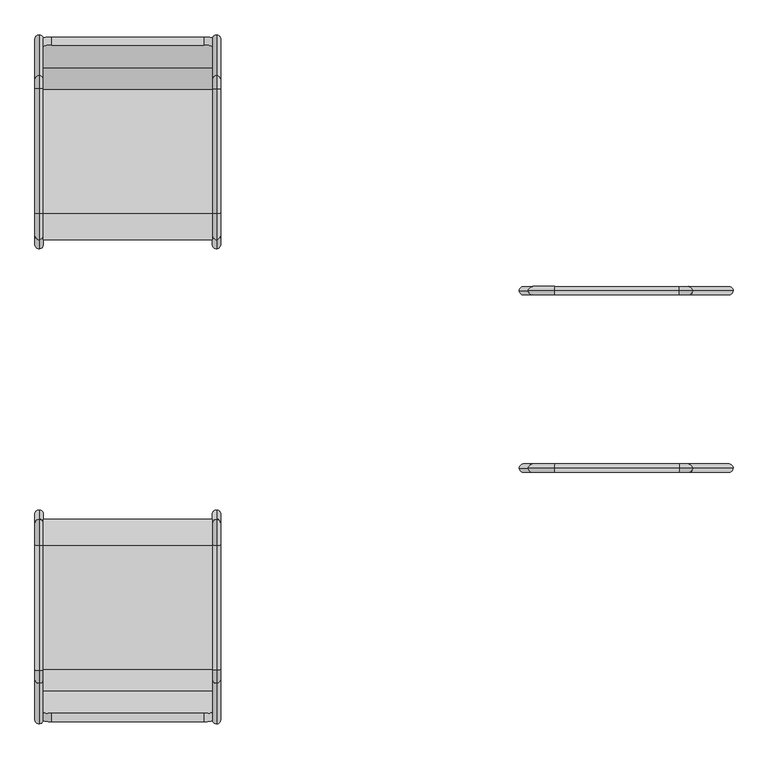
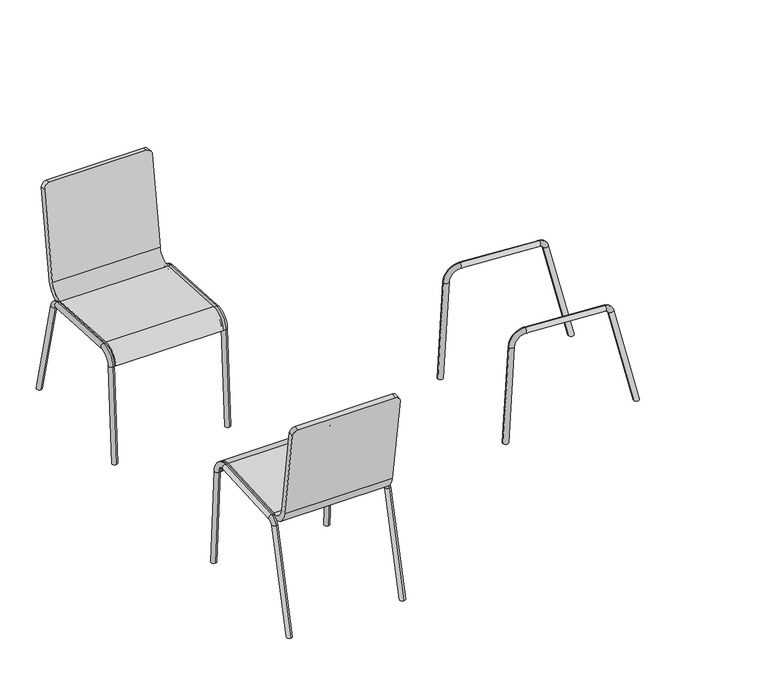
"""IFC4 building model written with IfcOpenShell, lengths in millimetres: furniture geometry."""

from ifc_helpers import new_model, si_unit, point, frame, origin, place, context, project, spatial, polyline, circle_curve, ellipse_curve, trimmed, source, transform, mapped, element, save
from ifc_brep_helpers import plane_surface, cylinder_surface, revolved_surface, advanced_brep


def furniture_c31c7c6f(model_context):
    return source(origin(), model_context, "Body", "AdvancedBrep", [
        advanced_brep(
        [(-273.9849702, -804.6938637, 0.0), (-273.9849702, -825.3061363, 0.0), (-263.9849702, -323.0385228, 0.0), (-273.9849702, -333.0554387, 0.0), (-283.9849702, -323.0385228, 0.0), (-273.9849702, -709.1722272, 383.1163586), (-273.9849702, -728.5781417, 387.9547965), (-273.9849702, -696.6509897, 414.4284246), (-273.9849702, -695.489162, 394.4621992), (-273.9849702, -398.2489468, 431.792335), (-273.9849702, -397.0871192, 411.8261096), (-273.9849702, -334.8647877, 375.3791418), (-273.9849702, -354.8310131, 374.2173141), (-273.9849702, -313.0554101, 0.5809138)],
        [
            (0, 1, ellipse_curve(frame((-273.9849702, -815.0, 0.0), z_axis=(0.0, 0.0, -1.0), x_axis=(0.0, -1.0, 0.0)), 10.3061363, 10.0)),
            (1, 0, ellipse_curve(frame((-273.9849702, -815.0, 0.0), z_axis=(0.0, 0.0, -1.0), x_axis=(0.0, -1.0, 0.0)), 10.3061363, 10.0)),
            (2, 3, ellipse_curve(frame((-273.9849702, -323.0385228, 0.0), z_axis=(0.0, 0.0, -1.0), x_axis=(0.0, -1.0, 0.0)), 10.0169159, 10.0)),
            (3, 4, ellipse_curve(frame((-273.9849702, -323.0385228, 0.0), z_axis=(0.0, 0.0, -1.0), x_axis=(0.0, -1.0, 0.0)), 10.0169159, 10.0)),
            (4, 2),
            (5, 0),
            (1, 6),
            (6, 5, circle_curve(frame((-273.9849702, -718.8751844, 385.5355776), z_axis=(0.0, -0.24192189559966623, -0.9702957262759968), x_axis=(0.0, -0.9702957262759968, 0.24192189559966623)), 10.0)),
            (5, 6, circle_curve(frame((-273.9849702, -718.8751844, 385.5355776), z_axis=(0.0, -0.24192189559966623, -0.9702957262759968), x_axis=(0.0, -0.9702957262759968, 0.24192189559966623)), 10.0)),
            (6, 7, circle_curve(frame((-273.9849702, -694.6177913, 379.4875302), z_axis=(-1.0, 0.0, 0.0), x_axis=(0.0, -0.9702957262759969, 0.2419218955996659)), 35.0)),
            (7, 8, circle_curve(frame((-273.9849702, -696.0700758, 404.4453119), z_axis=(0.0, -0.9983112697039765, -0.05809138302738456), x_axis=(0.0, -0.05809138302738456, 0.9983112697039765)), 10.0)),
            (8, 5, circle_curve(frame((-273.9849702, -694.6177913, 379.4875302), z_axis=(1.0, 0.0, 0.0), x_axis=(0.0, -0.9702957262759969, 0.2419218955996659)), 15.0)),
            (8, 7, circle_curve(frame((-273.9849702, -696.0700758, 404.4453119), z_axis=(0.0, -0.998311269703977, -0.05809138302737549), x_axis=(0.0, -0.05809138302737549, 0.998311269703977)), 10.0)),
            (7, 9),
            (9, 10, circle_curve(frame((-273.9849702, -397.668033, 421.8092223), z_axis=(0.0, -0.9983112697039764, -0.058091383027386895), x_axis=(0.0, -0.058091383027386895, 0.9983112697039764)), 10.0)),
            (10, 8),
            (10, 9, circle_curve(frame((-273.9849702, -397.668033, 421.8092223), z_axis=(0.0, -0.9983112697039764, -0.058091383027386895), x_axis=(0.0, -0.058091383027386895, 0.9983112697039764)), 10.0)),
            (9, 11, circle_curve(frame((-273.9849702, -394.7634639, 371.8936588), z_axis=(-1.0, 0.0, 0.0), x_axis=(0.0, -0.05809138302738633, 0.9983112697039764)), 60.0)),
            (11, 12, circle_curve(frame((-273.9849702, -344.8479004, 374.7982279), z_axis=(0.0, -0.05809138302739081, 0.9983112697039762), x_axis=(0.0, 0.9983112697039762, 0.05809138302739081)), 10.0)),
            (12, 10, circle_curve(frame((-273.9849702, -394.7634639, 371.8936588), z_axis=(1.0, 0.0, 0.0), x_axis=(0.0, -0.05809138302738633, 0.9983112697039764)), 40.0)),
            (12, 11, circle_curve(frame((-273.9849702, -344.8479004, 374.7982279), z_axis=(0.0, -0.05809138302739125, 0.9983112697039761), x_axis=(0.0, 0.9983112697039761, 0.05809138302739125)), 10.0)),
            (4, 13, circle_curve(frame((-273.9849702, -323.0385228, 0.0), z_axis=(0.0, 0.058091383027392335, -0.9983112697039761), x_axis=(0.0, 0.9983112697039761, 0.058091383027392335)), 10.0)),
            (13, 2, circle_curve(frame((-273.9849702, -323.0385228, 0.0), z_axis=(0.0, 0.058091383027392335, -0.9983112697039761), x_axis=(0.0, 0.9983112697039761, 0.058091383027392335)), 10.0)),
            (11, 13),
            (3, 12),
        ],
        [
            plane_surface(frame((-236.564671, -850.4463822, 0.0), z_axis=(0.0, 0.0, -1.0), x_axis=(-1.0, 0.0, 0.0))),
            cylinder_surface(frame((-273.9849702, -817.6101503, -10.4687411), z_axis=(0.0, -0.24192189559966623, -0.9702957262759968), x_axis=(0.0, -0.9702957262759968, 0.24192189559966623)), 10.0),
            revolved_surface(trimmed(ellipse_curve(frame((-273.9849702, -718.8751844, 385.5355776), z_axis=(0.0, 0.2419218955996659, 0.9702957262759969), x_axis=(0.0, -0.9702957262759969, 0.2419218955996659)), 10.0, 10.0), [point((-273.9849702, -709.1722272, 383.1163586))], [point((-273.9849702, -728.5781417, 387.9547965))], True, "CARTESIAN"), (-293.9849702, -694.6177913, 379.4875302), (1.0, 0.0, 0.0)),
            revolved_surface(trimmed(ellipse_curve(frame((-273.9849702, -718.8751844, 385.5355776), z_axis=(0.0, 0.2419218955996659, 0.9702957262759969), x_axis=(0.0, -0.9702957262759969, 0.2419218955996659)), 10.0, 10.0), [point((-273.9849702, -728.5781417, 387.9547965))], [point((-273.9849702, -709.1722272, 383.1163586))], True, "CARTESIAN"), (-293.9849702, -694.6177913, 379.4875302), (1.0, 0.0, 0.0)),
            cylinder_surface(frame((-273.9849702, -696.0700758, 404.4453119), z_axis=(0.0, -0.9983112697039764, -0.058091383027386895), x_axis=(0.0, -0.058091383027386895, 0.9983112697039764)), 10.0),
            revolved_surface(trimmed(ellipse_curve(frame((-273.9849702, -397.668033, 421.8092223), z_axis=(0.0, 0.9983112697039764, 0.05809138302738631), x_axis=(0.0, -0.05809138302738631, 0.9983112697039764)), 10.0, 10.0), [point((-273.9849702, -397.0871192, 411.8261096))], [point((-273.9849702, -398.2489468, 431.792335))], True, "CARTESIAN"), (-293.9849702, -394.7634639, 371.8936588), (1.0, 0.0, 0.0)),
            revolved_surface(trimmed(ellipse_curve(frame((-273.9849702, -397.668033, 421.8092223), z_axis=(0.0, 0.9983112697039764, 0.05809138302738631), x_axis=(0.0, -0.05809138302738631, 0.9983112697039764)), 10.0, 10.0), [point((-273.9849702, -398.2489468, 431.792335))], [point((-273.9849702, -397.0871192, 411.8261096))], True, "CARTESIAN"), (-293.9849702, -394.7634639, 371.8936588), (1.0, 0.0, 0.0)),
            plane_surface(frame((-293.9849702, -323.0385228, 0.0), z_axis=(0.0, 0.058091383027392335, -0.9983112697039761), x_axis=(1.0, 0.0, 0.0))),
            cylinder_surface(frame((-273.9849702, -344.8479004, 374.7982279), z_axis=(0.0, -0.058091383027392335, 0.9983112697039761), x_axis=(0.0, 0.9983112697039761, 0.058091383027392335)), 10.0),
        ],
        [
            (0, [[1, 2]]),
            (0, [[3, 4, 5]]),
            (1, [[6, -2, 7, 8]]),
            (1, [[-7, -1, -6, 9]]),
            (2, [[10, 11, 12, -8]]),
            (3, [[-12, 13, -10, -9]]),
            (4, [[14, 15, 16, -11]]),
            (4, [[-16, 17, -14, -13]]),
            (5, [[18, 19, 20, -15]]),
            (6, [[-20, 21, -18, -17]]),
            (7, [[-5, 22, 23]]),
            (8, [[24, -22, -4, 25, -19]]),
            (8, [[-25, -3, -23, -24, -21]]),
        ],
    ),
        advanced_brep(
        [(-689.1443717, -323.0385228, 0.0), (-709.1443717, -323.0385228, 0.0), (-699.1443717, -313.0554101, 0.5809138), (-699.1443717, -709.1722272, 383.1163586), (-699.1443717, -804.6938637, 0.0), (-699.1443717, -825.3061363, 0.0), (-699.1443717, -728.5781417, 387.9547965), (-699.1443717, -333.0554387, 0.0), (-699.1443717, -696.6509897, 414.4284246), (-699.1443717, -398.2489468, 431.792335), (-699.1443717, -397.0871192, 411.8261096), (-699.1443717, -695.489162, 394.4621992), (-699.1443717, -334.8647877, 375.3791418), (-699.1443717, -354.8310131, 374.2173141)],
        [
            (0, 1),
            (1, 2, circle_curve(frame((-699.1443717, -323.0385228, 0.0), z_axis=(0.0, 0.058091383027392335, -0.9983112697039761), x_axis=(0.0, 0.9983112697039761, 0.058091383027392335)), 10.0)),
            (2, 0, circle_curve(frame((-699.1443717, -323.0385228, 0.0), z_axis=(0.0, 0.058091383027392335, -0.9983112697039761), x_axis=(0.0, 0.9983112697039761, 0.058091383027392335)), 10.0)),
            (3, 4),
            (4, 5, ellipse_curve(frame((-699.1443717, -815.0, 0.0), z_axis=(0.0, 0.0, 1.0), x_axis=(0.0, -1.0, 0.0)), 10.3061363, 10.0)),
            (5, 6),
            (6, 3, circle_curve(frame((-699.1443717, -718.8751844, 385.5355776), z_axis=(0.0, -0.24192189559966623, -0.9702957262759968), x_axis=(0.0, -0.9702957262759968, 0.24192189559966623)), 10.0)),
            (5, 4, ellipse_curve(frame((-699.1443717, -815.0, 0.0), z_axis=(0.0, 0.0, 1.0), x_axis=(0.0, -1.0, 0.0)), 10.3061363, 10.0)),
            (3, 6, circle_curve(frame((-699.1443717, -718.8751844, 385.5355776), z_axis=(0.0, -0.24192189559966623, -0.9702957262759968), x_axis=(0.0, -0.9702957262759968, 0.24192189559966623)), 10.0)),
            (0, 7, ellipse_curve(frame((-699.1443717, -323.0385228, 0.0), z_axis=(0.0, 0.0, -1.0), x_axis=(0.0, -1.0, 0.0)), 10.0169159, 10.0)),
            (7, 1, ellipse_curve(frame((-699.1443717, -323.0385228, 0.0), z_axis=(0.0, 0.0, -1.0), x_axis=(0.0, -1.0, 0.0)), 10.0169159, 10.0)),
            (8, 9),
            (9, 10, circle_curve(frame((-699.1443717, -397.668033, 421.8092223), z_axis=(0.0, -0.9983112697039764, -0.058091383027386895), x_axis=(0.0, -0.058091383027386895, 0.9983112697039764)), 10.0)),
            (10, 11),
            (11, 8, circle_curve(frame((-699.1443717, -696.0700758, 404.4453119), z_axis=(0.0, 0.9983112697039764, 0.058091383027386895), x_axis=(0.0, -0.058091383027386895, 0.9983112697039764)), 10.0)),
            (10, 9, circle_curve(frame((-699.1443717, -397.668033, 421.8092223), z_axis=(0.0, -0.9983112697039764, -0.058091383027386895), x_axis=(0.0, -0.058091383027386895, 0.9983112697039764)), 10.0)),
            (8, 11, circle_curve(frame((-699.1443717, -696.0700758, 404.4453119), z_axis=(0.0, 0.9983112697039764, 0.058091383027386895), x_axis=(0.0, -0.058091383027386895, 0.9983112697039764)), 10.0)),
            (9, 12, circle_curve(frame((-699.1443717, -394.7634639, 371.8936588), z_axis=(-1.0, 0.0, 0.0), x_axis=(0.0, -0.05809138302738633, 0.9983112697039764)), 60.0)),
            (12, 13, circle_curve(frame((-699.1443717, -344.8479004, 374.7982279), z_axis=(0.0, -0.058091383027391474, 0.9983112697039761), x_axis=(0.0, 0.9983112697039761, 0.058091383027391474)), 10.0)),
            (13, 10, circle_curve(frame((-699.1443717, -394.7634639, 371.8936588), z_axis=(1.0, 0.0, 0.0), x_axis=(0.0, -0.05809138302738633, 0.9983112697039764)), 40.0)),
            (13, 12, circle_curve(frame((-699.1443717, -344.8479004, 374.7982279), z_axis=(0.0, -0.05809138302739081, 0.9983112697039762), x_axis=(0.0, 0.9983112697039762, 0.05809138302739081)), 10.0)),
            (12, 2),
            (7, 13),
            (6, 8, circle_curve(frame((-699.1443717, -694.6177913, 379.4875302), z_axis=(-1.0, 0.0, 0.0), x_axis=(0.0, -0.9702957262759969, 0.2419218955996659)), 35.0)),
            (11, 3, circle_curve(frame((-699.1443717, -694.6177913, 379.4875302), z_axis=(1.0, 0.0, 0.0), x_axis=(0.0, -0.9702957262759969, 0.2419218955996659)), 15.0)),
        ],
        [
            plane_surface(frame((-679.1443717, -323.0385228, 0.0), z_axis=(0.0, 0.058091383027392335, -0.9983112697039761), x_axis=(-1.0, 0.0, 0.0))),
            cylinder_surface(frame((-699.1443717, -817.6101503, -10.4687411), z_axis=(0.0, -0.24192189559966623, -0.9702957262759968), x_axis=(0.0, -0.9702957262759968, 0.24192189559966623)), 10.0),
            plane_surface(frame((-236.564671, -850.4463822, 0.0), z_axis=(0.0, 0.0, -1.0), x_axis=(-1.0, 0.0, 0.0))),
            cylinder_surface(frame((-699.1443717, -696.0700758, 404.4453119), z_axis=(0.0, -0.9983112697039764, -0.058091383027386895), x_axis=(0.0, -0.058091383027386895, 0.9983112697039764)), 10.0),
            revolved_surface(trimmed(ellipse_curve(frame((-699.1443717, -397.668033, 421.8092223), z_axis=(0.0, 0.9983112697039764, 0.05809138302738631), x_axis=(0.0, -0.05809138302738631, 0.9983112697039764)), 10.0, 10.0), [point((-699.1443717, -397.0871192, 411.8261096))], [point((-699.1443717, -398.2489468, 431.792335))], True, "CARTESIAN"), (-679.1443717, -394.7634639, 371.8936588), (1.0, 0.0, 0.0)),
            revolved_surface(trimmed(ellipse_curve(frame((-699.1443717, -397.668033, 421.8092223), z_axis=(0.0, 0.9983112697039764, 0.05809138302738631), x_axis=(0.0, -0.05809138302738631, 0.9983112697039764)), 10.0, 10.0), [point((-699.1443717, -398.2489468, 431.792335))], [point((-699.1443717, -397.0871192, 411.8261096))], True, "CARTESIAN"), (-679.1443717, -394.7634639, 371.8936588), (1.0, 0.0, 0.0)),
            cylinder_surface(frame((-699.1443717, -344.8479004, 374.7982279), z_axis=(0.0, -0.058091383027392335, 0.9983112697039761), x_axis=(0.0, 0.9983112697039761, 0.058091383027392335)), 10.0),
            revolved_surface(trimmed(ellipse_curve(frame((-699.1443717, -718.8751844, 385.5355776), z_axis=(0.0, 0.2419218955996659, 0.9702957262759969), x_axis=(0.0, -0.9702957262759969, 0.2419218955996659)), 10.0, 10.0), [point((-699.1443717, -709.1722272, 383.1163586))], [point((-699.1443717, -728.5781417, 387.9547965))], True, "CARTESIAN"), (-679.1443717, -694.6177913, 379.4875302), (1.0, 0.0, 0.0)),
            revolved_surface(trimmed(ellipse_curve(frame((-699.1443717, -718.8751844, 385.5355776), z_axis=(0.0, 0.2419218955996659, 0.9702957262759969), x_axis=(0.0, -0.9702957262759969, 0.2419218955996659)), 10.0, 10.0), [point((-699.1443717, -728.5781417, 387.9547965))], [point((-699.1443717, -709.1722272, 383.1163586))], True, "CARTESIAN"), (-679.1443717, -694.6177913, 379.4875302), (1.0, 0.0, 0.0)),
        ],
        [
            (0, [[1, 2, 3]]),
            (1, [[4, 5, 6, 7]]),
            (1, [[-6, 8, -4, 9]]),
            (2, [[-8, -5]]),
            (2, [[10, 11, -1]]),
            (3, [[12, 13, 14, 15]]),
            (3, [[-14, 16, -12, 17]]),
            (4, [[18, 19, 20, -13]]),
            (5, [[-20, 21, -18, -16]]),
            (6, [[22, -2, -11, 23, -19]]),
            (6, [[-23, -10, -3, -22, -21]]),
            (7, [[24, -15, 25, -7]]),
            (8, [[-25, -17, -24, -9]]),
        ],
    ),
        advanced_brep(
        [(-284.064671, -694.2901891, 414.5657988), (-284.064671, -746.6455514, 457.0908917), (-284.064671, -797.5017557, 797.3777006), (-284.064671, -817.282073, 794.4215124), (-284.064671, -766.4258686, 454.1347035), (-284.064671, -693.1283614, 394.5995734), (-284.064671, -397.0871192, 411.8261096), (-284.064671, -354.8310131, 374.2173141), (-284.064671, -334.8647877, 375.3791418), (-284.064671, -398.2489468, 431.792335), (-689.064671, -694.2901891, 414.5657988), (-689.064671, -398.2489468, 431.792335), (-689.064671, -334.8647877, 375.3791418), (-689.064671, -354.8310131, 374.2173141), (-689.064671, -397.0871192, 411.8261096), (-689.064671, -693.1283614, 394.5995734), (-689.064671, -766.4258686, 454.1347035), (-689.064671, -817.282073, 794.4215124), (-689.064671, -797.5017557, 797.3777006), (-689.064671, -746.6455514, 457.0908917), (-304.064671, -820.2382612, 814.2018297), (-669.064671, -820.2382612, 814.2018297), (-304.064671, -800.4579439, 817.1580179), (-669.064671, -800.4579439, 817.1580179)],
        [
            (0, 1, circle_curve(frame((-284.064671, -697.1947582, 464.4813623), z_axis=(-1.0, 0.0, 0.0), x_axis=(0.0, -1.0, 0.0)), 50.0)),
            (1, 2),
            (2, 3),
            (3, 4),
            (4, 5, circle_curve(frame((-284.064671, -697.1947582, 464.4813623), z_axis=(1.0, 0.0, 0.0), x_axis=(0.0, -1.0, 0.0)), 70.0)),
            (5, 6),
            (6, 7, circle_curve(frame((-284.064671, -394.7634639, 371.8936588), z_axis=(-1.0, 0.0, 0.0), x_axis=(0.0, -1.0, 0.0)), 40.0)),
            (7, 8),
            (8, 9, circle_curve(frame((-284.064671, -394.7634639, 371.8936588), z_axis=(1.0, 0.0, 0.0), x_axis=(0.0, -1.0, 0.0)), 60.0)),
            (9, 0),
            (10, 11),
            (11, 12, circle_curve(frame((-689.064671, -394.7634639, 371.8936588), z_axis=(-1.0, 0.0, 0.0), x_axis=(0.0, -1.0, 0.0)), 60.0)),
            (12, 13),
            (13, 14, circle_curve(frame((-689.064671, -394.7634639, 371.8936588), z_axis=(1.0, 0.0, 0.0), x_axis=(0.0, -1.0, 0.0)), 40.0)),
            (14, 15),
            (15, 16, circle_curve(frame((-689.064671, -697.1947582, 464.4813623), z_axis=(-1.0, 0.0, 0.0), x_axis=(0.0, -1.0, 0.0)), 70.0)),
            (16, 17),
            (17, 18),
            (18, 19),
            (19, 10, circle_curve(frame((-689.064671, -697.1947582, 464.4813623), z_axis=(1.0, 0.0, 0.0), x_axis=(0.0, -1.0, 0.0)), 50.0)),
            (9, 11),
            (10, 0),
            (8, 12),
            (7, 13),
            (6, 14),
            (5, 15),
            (4, 16),
            (3, 20, circle_curve(frame((-304.064671, -817.282073, 794.4215124), z_axis=(0.0, -0.9890158633619166, -0.14780941112961252), x_axis=(-1.0, 0.0, 0.0)), 20.0)),
            (20, 21),
            (21, 17, circle_curve(frame((-669.064671, -817.282073, 794.4215124), z_axis=(0.0, -0.9890158633619166, -0.14780941112961252), x_axis=(1.0, 0.0, 0.0)), 20.0)),
            (20, 22),
            (22, 23),
            (23, 21),
            (18, 23, circle_curve(frame((-669.064671, -797.5017557, 797.3777006), z_axis=(0.0, 0.9890158633619166, 0.14780941112961252), x_axis=(1.0, 0.0, 0.0)), 20.0)),
            (22, 2, circle_curve(frame((-304.064671, -797.5017557, 797.3777006), z_axis=(0.0, 0.9890158633619166, 0.14780941112961252), x_axis=(-1.0, 0.0, 0.0)), 20.0)),
            (1, 19),
        ],
        [
            plane_surface(frame((-284.064671, -400.4940122, 431.6616954), z_axis=(1.0000000000000002, 0.0, 0.0), x_axis=(0.0, 0.9983112697039764, 0.05809138302738736))),
            plane_surface(frame((-689.064671, -400.4940122, 431.6616954), z_axis=(-1.0000000000000002, 0.0, 0.0), x_axis=(0.0, -0.9983112697039764, -0.05809138302738736))),
            plane_surface(frame((-284.064671, -694.2901891, 414.5657988), z_axis=(0.0, -0.05809138302738736, 0.9983112697039764), x_axis=(-1.0, 0.0, 0.0))),
            cylinder_surface(frame((-689.064671, -394.7634639, 371.8936588), z_axis=(1.0, 0.0, 0.0), x_axis=(0.0, -1.0, 0.0)), 60.0),
            plane_surface(frame((-284.064671, -334.8647877, 375.3791418), z_axis=(0.0, 0.058091383027390926, -0.9983112697039762), x_axis=(-1.0, 0.0, 0.0))),
            revolved_surface(polyline([(-689.064671, -434.7634639, 371.8936588), (-284.064671, -434.7634639, 371.8936588)]), (-689.064671, -394.7634639, 371.8936588), (-1.0, 0.0, 0.0)),
            plane_surface(frame((-284.064671, -397.0871192, 411.8261096), z_axis=(0.0, 0.05809138302738756, -0.9983112697039763), x_axis=(-1.0, 0.0, 0.0))),
            cylinder_surface(frame((-689.064671, -697.1947582, 464.4813623), z_axis=(1.0, 0.0, 0.0), x_axis=(0.0, -1.0, 0.0)), 70.0),
            plane_surface(frame((-284.064671, -766.4258686, 454.1347035), z_axis=(0.0, -0.9890158633619166, -0.1478094111296125), x_axis=(-1.0, 0.0, 0.0))),
            plane_surface(frame((-284.064671, -820.2382612, 814.2018297), z_axis=(0.0, -0.14780941112961524, 0.9890158633619162), x_axis=(-1.0, 0.0, 0.0))),
            plane_surface(frame((-284.064671, -800.4579439, 817.1580179), z_axis=(0.0, 0.9890158633619166, 0.14780941112961254), x_axis=(-1.0, 0.0, 0.0))),
            revolved_surface(polyline([(-689.064671, -747.1947582, 464.4813623), (-284.064671, -747.1947582, 464.4813623)]), (-689.064671, -697.1947582, 464.4813623), (-1.0, 0.0, 0.0)),
            cylinder_surface(frame((-669.064671, -797.5017557, 797.3777006), z_axis=(0.0, 0.9890158633619166, 0.14780941112961252), x_axis=(1.0, 0.0, 0.0)), 20.0),
            cylinder_surface(frame((-304.064671, -797.5017557, 797.3777006), z_axis=(0.0, 0.9890158633619166, 0.14780941112961252), x_axis=(-1.0, 0.0, 0.0)), 20.0),
        ],
        [
            (0, [[1, 2, 3, 4, 5, 6, 7, 8, 9, 10]]),
            (1, [[11, 12, 13, 14, 15, 16, 17, 18, 19, 20]]),
            (2, [[21, -11, 22, -10]]),
            (3, [[23, -12, -21, -9]]),
            (4, [[24, -13, -23, -8]]),
            (5, [[25, -14, -24, -7]]),
            (6, [[26, -15, -25, -6]]),
            (7, [[27, -16, -26, -5]]),
            (8, [[-4, 28, 29, 30, -17, -27]]),
            (9, [[31, 32, 33, -29]]),
            (10, [[-19, 34, -32, 35, -2, 36]]),
            (11, [[-22, -20, -36, -1]]),
            (12, [[-30, -33, -34, -18]]),
            (13, [[-35, -31, -28, -3]]),
        ],
    ),
        advanced_brep(
        [(-273.9849702, 804.6938637, 0.0), (-273.9849702, 825.3061363, 0.0), (-263.9849702, 323.0385228, 0.0), (-283.9849702, 323.0385228, 0.0), (-273.9849702, 333.0554387, 0.0), (-273.9849702, 709.1722272, 383.1163586), (-273.9849702, 728.5781417, 387.9547965), (-273.9849702, 695.489162, 394.4621992), (-273.9849702, 696.6509897, 414.4284246), (-273.9849702, 397.0871192, 411.8261096), (-273.9849702, 398.2489468, 431.792335), (-273.9849702, 354.8310131, 374.2173141), (-273.9849702, 334.8647877, 375.3791418), (-273.9849702, 313.0554101, 0.5809138)],
        [
            (0, 1, ellipse_curve(frame((-273.9849702, 815.0, 0.0), z_axis=(0.0, 0.0, -1.0), x_axis=(0.0, 1.0, 0.0)), 10.3061363, 10.0)),
            (1, 0, ellipse_curve(frame((-273.9849702, 815.0, 0.0), z_axis=(0.0, 0.0, -1.0), x_axis=(0.0, 1.0, 0.0)), 10.3061363, 10.0)),
            (2, 3),
            (3, 4, ellipse_curve(frame((-273.9849702, 323.0385228, 0.0), z_axis=(0.0, 0.0, -1.0), x_axis=(0.0, 1.0, 0.0)), 10.0169159, 10.0)),
            (4, 2, ellipse_curve(frame((-273.9849702, 323.0385228, 0.0), z_axis=(0.0, 0.0, -1.0), x_axis=(0.0, 1.0, 0.0)), 10.0169159, 10.0)),
            (5, 6, circle_curve(frame((-273.9849702, 718.8751844, 385.5355776), z_axis=(0.0, 0.24192189559966623, -0.9702957262759968), x_axis=(0.0, 0.9702957262759968, 0.24192189559966623)), 10.0)),
            (6, 1),
            (0, 5),
            (6, 5, circle_curve(frame((-273.9849702, 718.8751844, 385.5355776), z_axis=(0.0, 0.24192189559966623, -0.9702957262759968), x_axis=(0.0, 0.9702957262759968, 0.24192189559966623)), 10.0)),
            (5, 7, circle_curve(frame((-273.9849702, 694.6177913, 379.4875302), z_axis=(1.0, 0.0, 0.0), x_axis=(0.0, 0.9702957262759969, 0.2419218955996659)), 15.0)),
            (7, 8, circle_curve(frame((-273.9849702, 696.0700758, 404.4453119), z_axis=(0.0, 0.998311269703977, -0.058091383027376764), x_axis=(0.0, 0.058091383027376764, 0.998311269703977)), 10.0)),
            (8, 6, circle_curve(frame((-273.9849702, 694.6177913, 379.4875302), z_axis=(-1.0, 0.0, 0.0), x_axis=(0.0, 0.9702957262759969, 0.2419218955996659)), 35.0)),
            (8, 7, circle_curve(frame((-273.9849702, 696.0700758, 404.4453119), z_axis=(0.0, 0.9983112697039765, -0.05809138302738498), x_axis=(0.0, 0.05809138302738498, 0.9983112697039765)), 10.0)),
            (7, 9),
            (9, 10, circle_curve(frame((-273.9849702, 397.668033, 421.8092223), z_axis=(0.0, 0.9983112697039764, -0.058091383027386895), x_axis=(0.0, 0.058091383027386895, 0.9983112697039764)), 10.0)),
            (10, 8),
            (10, 9, circle_curve(frame((-273.9849702, 397.668033, 421.8092223), z_axis=(0.0, 0.9983112697039764, -0.058091383027386895), x_axis=(0.0, 0.058091383027386895, 0.9983112697039764)), 10.0)),
            (9, 11, circle_curve(frame((-273.9849702, 394.7634639, 371.8936588), z_axis=(1.0, 0.0, 0.0), x_axis=(0.0, 0.05809138302738633, 0.9983112697039764)), 40.0)),
            (11, 12, circle_curve(frame((-273.9849702, 344.8479004, 374.7982279), z_axis=(0.0, 0.058091383027391474, 0.9983112697039761), x_axis=(0.0, -0.9983112697039761, 0.058091383027391474)), 10.0)),
            (12, 10, circle_curve(frame((-273.9849702, 394.7634639, 371.8936588), z_axis=(-1.0, 0.0, 0.0), x_axis=(0.0, 0.05809138302738633, 0.9983112697039764)), 60.0)),
            (12, 11, circle_curve(frame((-273.9849702, 344.8479004, 374.7982279), z_axis=(0.0, 0.05809138302739081, 0.9983112697039762), x_axis=(0.0, -0.9983112697039762, 0.05809138302739081)), 10.0)),
            (2, 13, circle_curve(frame((-273.9849702, 323.0385228, 0.0), z_axis=(0.0, -0.058091383027392335, -0.9983112697039761), x_axis=(0.0, -0.9983112697039761, 0.058091383027392335)), 10.0)),
            (13, 3, circle_curve(frame((-273.9849702, 323.0385228, 0.0), z_axis=(0.0, -0.058091383027392335, -0.9983112697039761), x_axis=(0.0, -0.9983112697039761, 0.058091383027392335)), 10.0)),
            (11, 4),
            (13, 12),
        ],
        [
            plane_surface(frame((-236.564671, 850.4463822, 0.0), z_axis=(0.0, 0.0, -1.0), x_axis=(-1.0, 0.0, 0.0))),
            cylinder_surface(frame((-273.9849702, 817.6101503, -10.4687411), z_axis=(0.0, 0.24192189559966623, -0.9702957262759968), x_axis=(0.0, 0.9702957262759968, 0.24192189559966623)), 10.0),
            revolved_surface(trimmed(ellipse_curve(frame((-273.9849702, 718.8751844, 385.5355776), z_axis=(0.0, 0.2419218955996659, -0.9702957262759969), x_axis=(0.0, 0.9702957262759969, 0.2419218955996659)), 10.0, 10.0), [point((-273.9849702, 709.1722272, 383.1163586))], [point((-273.9849702, 728.5781417, 387.9547965))], True, "CARTESIAN"), (-293.9849702, 694.6177913, 379.4875302), (1.0, 0.0, 0.0)),
            revolved_surface(trimmed(ellipse_curve(frame((-273.9849702, 718.8751844, 385.5355776), z_axis=(0.0, 0.2419218955996659, -0.9702957262759969), x_axis=(0.0, 0.9702957262759969, 0.2419218955996659)), 10.0, 10.0), [point((-273.9849702, 728.5781417, 387.9547965))], [point((-273.9849702, 709.1722272, 383.1163586))], True, "CARTESIAN"), (-293.9849702, 694.6177913, 379.4875302), (1.0, 0.0, 0.0)),
            cylinder_surface(frame((-273.9849702, 696.0700758, 404.4453119), z_axis=(0.0, 0.9983112697039764, -0.058091383027386895), x_axis=(0.0, 0.058091383027386895, 0.9983112697039764)), 10.0),
            revolved_surface(trimmed(ellipse_curve(frame((-273.9849702, 397.668033, 421.8092223), z_axis=(0.0, 0.9983112697039764, -0.05809138302738631), x_axis=(0.0, 0.05809138302738631, 0.9983112697039764)), 10.0, 10.0), [point((-273.9849702, 397.0871192, 411.8261096))], [point((-273.9849702, 398.2489468, 431.792335))], True, "CARTESIAN"), (-293.9849702, 394.7634639, 371.8936588), (1.0, 0.0, 0.0)),
            revolved_surface(trimmed(ellipse_curve(frame((-273.9849702, 397.668033, 421.8092223), z_axis=(0.0, 0.9983112697039764, -0.05809138302738631), x_axis=(0.0, 0.05809138302738631, 0.9983112697039764)), 10.0, 10.0), [point((-273.9849702, 398.2489468, 431.792335))], [point((-273.9849702, 397.0871192, 411.8261096))], True, "CARTESIAN"), (-293.9849702, 394.7634639, 371.8936588), (1.0, 0.0, 0.0)),
            plane_surface(frame((-293.9849702, 323.0385228, 0.0), z_axis=(0.0, -0.058091383027392335, -0.9983112697039761), x_axis=(1.0, 0.0, 0.0))),
            cylinder_surface(frame((-273.9849702, 344.8479004, 374.7982279), z_axis=(0.0, 0.058091383027392335, 0.9983112697039761), x_axis=(0.0, -0.9983112697039761, 0.058091383027392335)), 10.0),
        ],
        [
            (0, [[1, 2]]),
            (0, [[3, 4, 5]]),
            (1, [[6, 7, -1, 8]]),
            (1, [[9, -8, -2, -7]]),
            (2, [[-6, 10, 11, 12]]),
            (3, [[-9, -12, 13, -10]]),
            (4, [[-11, 14, 15, 16]]),
            (4, [[-13, -16, 17, -14]]),
            (5, [[-15, 18, 19, 20]]),
            (6, [[-17, -20, 21, -18]]),
            (7, [[22, 23, -3]]),
            (8, [[-19, 24, -4, -23, 25]]),
            (8, [[-21, -25, -22, -5, -24]]),
        ],
    ),
        advanced_brep(
        [(-689.1443717, 323.0385228, 0.0), (-699.1443717, 313.0554101, 0.5809138), (-709.1443717, 323.0385228, 0.0), (-699.1443717, 709.1722272, 383.1163586), (-699.1443717, 728.5781417, 387.9547965), (-699.1443717, 825.3061363, 0.0), (-699.1443717, 804.6938637, 0.0), (-699.1443717, 333.0554387, 0.0), (-699.1443717, 696.6509897, 414.4284246), (-699.1443717, 695.489162, 394.4621992), (-699.1443717, 397.0871192, 411.8261096), (-699.1443717, 398.2489468, 431.792335), (-699.1443717, 354.8310131, 374.2173141), (-699.1443717, 334.8647877, 375.3791418)],
        [
            (0, 1, circle_curve(frame((-699.1443717, 323.0385228, 0.0), z_axis=(0.0, -0.058091383027392335, -0.9983112697039761), x_axis=(0.0, -0.9983112697039761, 0.058091383027392335)), 10.0)),
            (1, 2, circle_curve(frame((-699.1443717, 323.0385228, 0.0), z_axis=(0.0, -0.058091383027392335, -0.9983112697039761), x_axis=(0.0, -0.9983112697039761, 0.058091383027392335)), 10.0)),
            (2, 0),
            (3, 4, circle_curve(frame((-699.1443717, 718.8751844, 385.5355776), z_axis=(0.0, 0.24192189559966623, -0.9702957262759968), x_axis=(0.0, 0.9702957262759968, 0.24192189559966623)), 10.0)),
            (4, 5),
            (5, 6, ellipse_curve(frame((-699.1443717, 815.0, 0.0), z_axis=(0.0, 0.0, 1.0), x_axis=(0.0, 1.0, 0.0)), 10.3061363, 10.0)),
            (6, 3),
            (4, 3, circle_curve(frame((-699.1443717, 718.8751844, 385.5355776), z_axis=(0.0, 0.24192189559966623, -0.9702957262759968), x_axis=(0.0, 0.9702957262759968, 0.24192189559966623)), 10.0)),
            (6, 5, ellipse_curve(frame((-699.1443717, 815.0, 0.0), z_axis=(0.0, 0.0, 1.0), x_axis=(0.0, 1.0, 0.0)), 10.3061363, 10.0)),
            (2, 7, ellipse_curve(frame((-699.1443717, 323.0385228, 0.0), z_axis=(0.0, 0.0, -1.0), x_axis=(0.0, 1.0, 0.0)), 10.0169159, 10.0)),
            (7, 0, ellipse_curve(frame((-699.1443717, 323.0385228, 0.0), z_axis=(0.0, 0.0, -1.0), x_axis=(0.0, 1.0, 0.0)), 10.0169159, 10.0)),
            (8, 9, circle_curve(frame((-699.1443717, 696.0700758, 404.4453119), z_axis=(0.0, -0.9983112697039764, 0.058091383027386895), x_axis=(0.0, 0.058091383027386895, 0.9983112697039764)), 10.0)),
            (9, 10),
            (10, 11, circle_curve(frame((-699.1443717, 397.668033, 421.8092223), z_axis=(0.0, 0.9983112697039764, -0.058091383027386895), x_axis=(0.0, 0.058091383027386895, 0.9983112697039764)), 10.0)),
            (11, 8),
            (9, 8, circle_curve(frame((-699.1443717, 696.0700758, 404.4453119), z_axis=(0.0, -0.9983112697039764, 0.058091383027386895), x_axis=(0.0, 0.058091383027386895, 0.9983112697039764)), 10.0)),
            (11, 10, circle_curve(frame((-699.1443717, 397.668033, 421.8092223), z_axis=(0.0, 0.9983112697039764, -0.058091383027386895), x_axis=(0.0, 0.058091383027386895, 0.9983112697039764)), 10.0)),
            (10, 12, circle_curve(frame((-699.1443717, 394.7634639, 371.8936588), z_axis=(1.0, 0.0, 0.0), x_axis=(0.0, 0.05809138302738633, 0.9983112697039764)), 40.0)),
            (12, 13, circle_curve(frame((-699.1443717, 344.8479004, 374.7982279), z_axis=(0.0, 0.058091383027391474, 0.9983112697039761), x_axis=(0.0, -0.9983112697039761, 0.058091383027391474)), 10.0)),
            (13, 11, circle_curve(frame((-699.1443717, 394.7634639, 371.8936588), z_axis=(-1.0, 0.0, 0.0), x_axis=(0.0, 0.05809138302738633, 0.9983112697039764)), 60.0)),
            (13, 12, circle_curve(frame((-699.1443717, 344.8479004, 374.7982279), z_axis=(0.0, 0.05809138302739081, 0.9983112697039762), x_axis=(0.0, -0.9983112697039762, 0.05809138302739081)), 10.0)),
            (12, 7),
            (1, 13),
            (3, 9, circle_curve(frame((-699.1443717, 694.6177913, 379.4875302), z_axis=(1.0, 0.0, 0.0), x_axis=(0.0, 0.9702957262759969, 0.2419218955996659)), 15.0)),
            (8, 4, circle_curve(frame((-699.1443717, 694.6177913, 379.4875302), z_axis=(-1.0, 0.0, 0.0), x_axis=(0.0, 0.9702957262759969, 0.2419218955996659)), 35.0)),
        ],
        [
            plane_surface(frame((-679.1443717, 323.0385228, 0.0), z_axis=(0.0, -0.058091383027392335, -0.9983112697039761), x_axis=(-1.0, 0.0, 0.0))),
            cylinder_surface(frame((-699.1443717, 817.6101503, -10.4687411), z_axis=(0.0, 0.24192189559966623, -0.9702957262759968), x_axis=(0.0, 0.9702957262759968, 0.24192189559966623)), 10.0),
            plane_surface(frame((-236.564671, 850.4463822, 0.0), z_axis=(0.0, 0.0, -1.0), x_axis=(-1.0, 0.0, 0.0))),
            cylinder_surface(frame((-699.1443717, 696.0700758, 404.4453119), z_axis=(0.0, 0.9983112697039764, -0.058091383027386895), x_axis=(0.0, 0.058091383027386895, 0.9983112697039764)), 10.0),
            revolved_surface(trimmed(ellipse_curve(frame((-699.1443717, 397.668033, 421.8092223), z_axis=(0.0, 0.9983112697039764, -0.05809138302738631), x_axis=(0.0, 0.05809138302738631, 0.9983112697039764)), 10.0, 10.0), [point((-699.1443717, 397.0871192, 411.8261096))], [point((-699.1443717, 398.2489468, 431.792335))], True, "CARTESIAN"), (-679.1443717, 394.7634639, 371.8936588), (1.0, 0.0, 0.0)),
            revolved_surface(trimmed(ellipse_curve(frame((-699.1443717, 397.668033, 421.8092223), z_axis=(0.0, 0.9983112697039764, -0.05809138302738631), x_axis=(0.0, 0.05809138302738631, 0.9983112697039764)), 10.0, 10.0), [point((-699.1443717, 398.2489468, 431.792335))], [point((-699.1443717, 397.0871192, 411.8261096))], True, "CARTESIAN"), (-679.1443717, 394.7634639, 371.8936588), (1.0, 0.0, 0.0)),
            cylinder_surface(frame((-699.1443717, 344.8479004, 374.7982279), z_axis=(0.0, 0.058091383027392335, 0.9983112697039761), x_axis=(0.0, -0.9983112697039761, 0.058091383027392335)), 10.0),
            revolved_surface(trimmed(ellipse_curve(frame((-699.1443717, 718.8751844, 385.5355776), z_axis=(0.0, 0.2419218955996659, -0.9702957262759969), x_axis=(0.0, 0.9702957262759969, 0.2419218955996659)), 10.0, 10.0), [point((-699.1443717, 709.1722272, 383.1163586))], [point((-699.1443717, 728.5781417, 387.9547965))], True, "CARTESIAN"), (-679.1443717, 694.6177913, 379.4875302), (1.0, 0.0, 0.0)),
            revolved_surface(trimmed(ellipse_curve(frame((-699.1443717, 718.8751844, 385.5355776), z_axis=(0.0, 0.2419218955996659, -0.9702957262759969), x_axis=(0.0, 0.9702957262759969, 0.2419218955996659)), 10.0, 10.0), [point((-699.1443717, 728.5781417, 387.9547965))], [point((-699.1443717, 709.1722272, 383.1163586))], True, "CARTESIAN"), (-679.1443717, 694.6177913, 379.4875302), (1.0, 0.0, 0.0)),
        ],
        [
            (0, [[1, 2, 3]]),
            (1, [[4, 5, 6, 7]]),
            (1, [[8, -7, 9, -5]]),
            (2, [[-3, 10, 11]]),
            (2, [[-6, -9]]),
            (3, [[12, 13, 14, 15]]),
            (3, [[16, -15, 17, -13]]),
            (4, [[-14, 18, 19, 20]]),
            (5, [[-17, -20, 21, -18]]),
            (6, [[-19, 22, -10, -2, 23]]),
            (6, [[-21, -23, -1, -11, -22]]),
            (7, [[-4, 24, -12, 25]]),
            (8, [[-8, -25, -16, -24]]),
        ],
    ),
        advanced_brep(
        [(-284.064671, 694.2901891, 414.5657988), (-284.064671, 398.2489468, 431.792335), (-284.064671, 334.8647877, 375.3791418), (-284.064671, 354.8310131, 374.2173141), (-284.064671, 397.0871192, 411.8261096), (-284.064671, 693.1283614, 394.5995734), (-284.064671, 766.4258686, 454.1347035), (-284.064671, 817.282073, 794.4215124), (-284.064671, 797.5017557, 797.3777006), (-284.064671, 746.6455514, 457.0908917), (-689.064671, 694.2901891, 414.5657988), (-689.064671, 746.6455514, 457.0908917), (-689.064671, 797.5017557, 797.3777006), (-689.064671, 817.282073, 794.4215124), (-689.064671, 766.4258686, 454.1347035), (-689.064671, 693.1283614, 394.5995734), (-689.064671, 397.0871192, 411.8261096), (-689.064671, 354.8310131, 374.2173141), (-689.064671, 334.8647877, 375.3791418), (-689.064671, 398.2489468, 431.792335), (-669.064671, 820.2382612, 814.2018297), (-304.064671, 820.2382612, 814.2018297), (-669.064671, 800.4579439, 817.1580179), (-304.064671, 800.4579439, 817.1580179)],
        [
            (0, 1),
            (1, 2, circle_curve(frame((-284.064671, 394.7634639, 371.8936588), z_axis=(1.0, 0.0, 0.0), x_axis=(0.0, 1.0, 0.0)), 60.0)),
            (2, 3),
            (3, 4, circle_curve(frame((-284.064671, 394.7634639, 371.8936588), z_axis=(-1.0, 0.0, 0.0), x_axis=(0.0, 1.0, 0.0)), 40.0)),
            (4, 5),
            (5, 6, circle_curve(frame((-284.064671, 697.1947582, 464.4813623), z_axis=(1.0, 0.0, 0.0), x_axis=(0.0, 1.0, 0.0)), 70.0)),
            (6, 7),
            (7, 8),
            (8, 9),
            (9, 0, circle_curve(frame((-284.064671, 697.1947582, 464.4813623), z_axis=(-1.0, 0.0, 0.0), x_axis=(0.0, 1.0, 0.0)), 50.0)),
            (10, 11, circle_curve(frame((-689.064671, 697.1947582, 464.4813623), z_axis=(1.0, 0.0, 0.0), x_axis=(0.0, 1.0, 0.0)), 50.0)),
            (11, 12),
            (12, 13),
            (13, 14),
            (14, 15, circle_curve(frame((-689.064671, 697.1947582, 464.4813623), z_axis=(-1.0, 0.0, 0.0), x_axis=(0.0, 1.0, 0.0)), 70.0)),
            (15, 16),
            (16, 17, circle_curve(frame((-689.064671, 394.7634639, 371.8936588), z_axis=(1.0, 0.0, 0.0), x_axis=(0.0, 1.0, 0.0)), 40.0)),
            (17, 18),
            (18, 19, circle_curve(frame((-689.064671, 394.7634639, 371.8936588), z_axis=(-1.0, 0.0, 0.0), x_axis=(0.0, 1.0, 0.0)), 60.0)),
            (19, 10),
            (0, 10),
            (19, 1),
            (18, 2),
            (17, 3),
            (16, 4),
            (15, 5),
            (14, 6),
            (13, 20, circle_curve(frame((-669.064671, 817.282073, 794.4215124), z_axis=(0.0, 0.9890158633619166, -0.14780941112961252), x_axis=(1.0, 0.0, 0.0)), 20.0)),
            (20, 21),
            (21, 7, circle_curve(frame((-304.064671, 817.282073, 794.4215124), z_axis=(0.0, 0.9890158633619166, -0.14780941112961252), x_axis=(-1.0, 0.0, 0.0)), 20.0)),
            (20, 22),
            (22, 23),
            (23, 21),
            (11, 9),
            (8, 23, circle_curve(frame((-304.064671, 797.5017557, 797.3777006), z_axis=(0.0, -0.9890158633619166, 0.14780941112961252), x_axis=(-1.0, 0.0, 0.0)), 20.0)),
            (22, 12, circle_curve(frame((-669.064671, 797.5017557, 797.3777006), z_axis=(0.0, -0.9890158633619166, 0.14780941112961252), x_axis=(1.0, 0.0, 0.0)), 20.0)),
        ],
        [
            plane_surface(frame((-284.064671, 400.4940122, 431.6616954), z_axis=(1.0000000000000002, 0.0, 0.0), x_axis=(0.0, -0.9983112697039764, 0.05809138302738736))),
            plane_surface(frame((-689.064671, 400.4940122, 431.6616954), z_axis=(-1.0000000000000002, 0.0, 0.0), x_axis=(0.0, 0.9983112697039764, -0.05809138302738736))),
            plane_surface(frame((-284.064671, 694.2901891, 414.5657988), z_axis=(0.0, 0.05809138302738736, 0.9983112697039764), x_axis=(-1.0, 0.0, 0.0))),
            cylinder_surface(frame((-689.064671, 394.7634639, 371.8936588), z_axis=(1.0, 0.0, 0.0), x_axis=(0.0, 1.0, 0.0)), 60.0),
            plane_surface(frame((-284.064671, 334.8647877, 375.3791418), z_axis=(0.0, -0.058091383027390926, -0.9983112697039762), x_axis=(-1.0, 0.0, 0.0))),
            revolved_surface(polyline([(-689.064671, 434.7634639, 371.8936588), (-284.064671, 434.7634639, 371.8936588)]), (-689.064671, 394.7634639, 371.8936588), (-1.0, 0.0, 0.0)),
            plane_surface(frame((-284.064671, 397.0871192, 411.8261096), z_axis=(0.0, -0.05809138302738756, -0.9983112697039763), x_axis=(-1.0, 0.0, 0.0))),
            cylinder_surface(frame((-689.064671, 697.1947582, 464.4813623), z_axis=(1.0, 0.0, 0.0), x_axis=(0.0, 1.0, 0.0)), 70.0),
            plane_surface(frame((-284.064671, 766.4258686, 454.1347035), z_axis=(0.0, 0.9890158633619166, -0.1478094111296125), x_axis=(-1.0, 0.0, 0.0))),
            plane_surface(frame((-284.064671, 820.2382612, 814.2018297), z_axis=(0.0, 0.14780941112961524, 0.9890158633619162), x_axis=(-1.0, 0.0, 0.0))),
            plane_surface(frame((-284.064671, 800.4579439, 817.1580179), z_axis=(0.0, -0.9890158633619166, 0.14780941112961254), x_axis=(-1.0, 0.0, 0.0))),
            revolved_surface(polyline([(-689.064671, 747.1947582, 464.4813623), (-284.064671, 747.1947582, 464.4813623)]), (-689.064671, 697.1947582, 464.4813623), (-1.0, 0.0, 0.0)),
            cylinder_surface(frame((-669.064671, 797.5017557, 797.3777006), z_axis=(0.0, -0.9890158633619166, 0.14780941112961252), x_axis=(1.0, 0.0, 0.0)), 20.0),
            cylinder_surface(frame((-304.064671, 797.5017557, 797.3777006), z_axis=(0.0, -0.9890158633619166, 0.14780941112961252), x_axis=(-1.0, 0.0, 0.0)), 20.0),
        ],
        [
            (0, [[1, 2, 3, 4, 5, 6, 7, 8, 9, 10]]),
            (1, [[11, 12, 13, 14, 15, 16, 17, 18, 19, 20]]),
            (2, [[-1, 21, -20, 22]]),
            (3, [[-2, -22, -19, 23]]),
            (4, [[-3, -23, -18, 24]]),
            (5, [[-4, -24, -17, 25]]),
            (6, [[-5, -25, -16, 26]]),
            (7, [[-6, -26, -15, 27]]),
            (8, [[-27, -14, 28, 29, 30, -7]]),
            (9, [[-29, 31, 32, 33]]),
            (10, [[34, -9, 35, -32, 36, -12]]),
            (11, [[-10, -34, -11, -21]]),
            (12, [[-13, -36, -31, -28]]),
            (13, [[-8, -30, -33, -35]]),
        ],
    ),
        advanced_brep(
        [(943.1291927, 212.5797007, 0.0), (963.7414653, 212.5797007, 0.0), (461.4738518, 222.5797007, 0.0), (471.4907677, 212.5797007, 0.0), (461.4738518, 202.5797007, 0.0), (847.6075562, 212.5797007, 383.1163586), (867.0134707, 212.5797007, 387.9547965), (835.0863187, 212.5797007, 414.4284246), (833.924491, 212.5797007, 394.4621992), (536.6842759, 212.5797007, 431.792335), (535.5224482, 212.5797007, 411.8261096), (473.3001167, 212.5797007, 375.3791418), (493.2663421, 212.5797007, 374.2173141), (451.4907391, 212.5797007, 0.5809138)],
        [
            (0, 1, ellipse_curve(frame((953.435329, 212.5797007, 0.0), z_axis=(0.0, 0.0, -1.0), x_axis=(1.0, 0.0, 0.0)), 10.3061363, 10.0)),
            (1, 0, ellipse_curve(frame((953.435329, 212.5797007, 0.0), z_axis=(0.0, 0.0, -1.0), x_axis=(1.0, 0.0, 0.0)), 10.3061363, 10.0)),
            (2, 3, ellipse_curve(frame((461.4738518, 212.5797007, 0.0), z_axis=(0.0, 0.0, -1.0), x_axis=(1.0, 0.0, 0.0)), 10.0169159, 10.0)),
            (3, 4, ellipse_curve(frame((461.4738518, 212.5797007, 0.0), z_axis=(0.0, 0.0, -1.0), x_axis=(1.0, 0.0, 0.0)), 10.0169159, 10.0)),
            (4, 2),
            (5, 0),
            (1, 6),
            (6, 5, circle_curve(frame((857.3105135, 212.5797007, 385.5355776), z_axis=(0.24192189559966623, 0.0, -0.9702957262759968), x_axis=(0.9702957262759968, 0.0, 0.24192189559966623)), 10.0)),
            (5, 6, circle_curve(frame((857.3105135, 212.5797007, 385.5355776), z_axis=(0.24192189559966623, 0.0, -0.9702957262759968), x_axis=(0.9702957262759968, 0.0, 0.24192189559966623)), 10.0)),
            (6, 7, circle_curve(frame((833.0531203, 212.5797007, 379.4875302), z_axis=(0.0, -1.0, 0.0), x_axis=(0.9702957262759969, 0.0, 0.2419218955996659)), 35.0)),
            (7, 8, circle_curve(frame((834.5054049, 212.5797007, 404.4453119), z_axis=(0.9983112697039765, 0.0, -0.05809138302738456), x_axis=(0.05809138302738456, 0.0, 0.9983112697039765)), 10.0)),
            (8, 5, circle_curve(frame((833.0531203, 212.5797007, 379.4875302), z_axis=(0.0, 1.0, 0.0), x_axis=(0.9702957262759969, 0.0, 0.2419218955996659)), 15.0)),
            (8, 7, circle_curve(frame((834.5054049, 212.5797007, 404.4453119), z_axis=(0.998311269703977, 0.0, -0.05809138302737549), x_axis=(0.05809138302737549, 0.0, 0.998311269703977)), 10.0)),
            (7, 9),
            (9, 10, circle_curve(frame((536.103362, 212.5797007, 421.8092223), z_axis=(0.9983112697039764, 0.0, -0.058091383027386895), x_axis=(0.058091383027386895, 0.0, 0.9983112697039764)), 10.0)),
            (10, 8),
            (10, 9, circle_curve(frame((536.103362, 212.5797007, 421.8092223), z_axis=(0.9983112697039764, 0.0, -0.058091383027386895), x_axis=(0.058091383027386895, 0.0, 0.9983112697039764)), 10.0)),
            (9, 11, circle_curve(frame((533.1987929, 212.5797007, 371.8936588), z_axis=(0.0, -1.0, 0.0), x_axis=(0.05809138302738633, 0.0, 0.9983112697039764)), 60.0)),
            (11, 12, circle_curve(frame((483.2832294, 212.5797007, 374.7982279), z_axis=(0.05809138302739081, 0.0, 0.9983112697039762), x_axis=(-0.9983112697039762, 0.0, 0.05809138302739081)), 10.0)),
            (12, 10, circle_curve(frame((533.1987929, 212.5797007, 371.8936588), z_axis=(0.0, 1.0, 0.0), x_axis=(0.05809138302738633, 0.0, 0.9983112697039764)), 40.0)),
            (12, 11, circle_curve(frame((483.2832294, 212.5797007, 374.7982279), z_axis=(0.05809138302739125, 0.0, 0.9983112697039761), x_axis=(-0.9983112697039761, 0.0, 0.05809138302739125)), 10.0)),
            (4, 13, circle_curve(frame((461.4738518, 212.5797007, 0.0), z_axis=(-0.058091383027392335, 0.0, -0.9983112697039761), x_axis=(-0.9983112697039761, 0.0, 0.058091383027392335)), 10.0)),
            (13, 2, circle_curve(frame((461.4738518, 212.5797007, 0.0), z_axis=(-0.058091383027392335, 0.0, -0.9983112697039761), x_axis=(-0.9983112697039761, 0.0, 0.058091383027392335)), 10.0)),
            (11, 13),
            (3, 12),
        ],
        [
            plane_surface(frame((988.8817112, 250.0, 0.0), z_axis=(0.0, 0.0, -1.0), x_axis=(0.0, -1.0, 0.0))),
            cylinder_surface(frame((956.0454793, 212.5797007, -10.4687411), z_axis=(0.24192189559966623, 0.0, -0.9702957262759968), x_axis=(0.9702957262759968, 0.0, 0.24192189559966623)), 10.0),
            revolved_surface(trimmed(ellipse_curve(frame((857.3105135, 212.5797007, 385.5355776), z_axis=(-0.2419218955996659, 0.0, 0.9702957262759969), x_axis=(0.9702957262759969, 0.0, 0.2419218955996659)), 10.0, 10.0), [point((847.6075562, 212.5797007, 383.1163586))], [point((867.0134707, 212.5797007, 387.9547965))], True, "CARTESIAN"), (833.0531203, 192.5797007, 379.4875302), (0.0, 1.0, 0.0)),
            revolved_surface(trimmed(ellipse_curve(frame((857.3105135, 212.5797007, 385.5355776), z_axis=(-0.2419218955996659, 0.0, 0.9702957262759969), x_axis=(0.9702957262759969, 0.0, 0.2419218955996659)), 10.0, 10.0), [point((867.0134707, 212.5797007, 387.9547965))], [point((847.6075562, 212.5797007, 383.1163586))], True, "CARTESIAN"), (833.0531203, 192.5797007, 379.4875302), (0.0, 1.0, 0.0)),
            cylinder_surface(frame((834.5054049, 212.5797007, 404.4453119), z_axis=(0.9983112697039764, 0.0, -0.058091383027386895), x_axis=(0.058091383027386895, 0.0, 0.9983112697039764)), 10.0),
            revolved_surface(trimmed(ellipse_curve(frame((536.103362, 212.5797007, 421.8092223), z_axis=(-0.9983112697039764, 0.0, 0.05809138302738631), x_axis=(0.05809138302738631, 0.0, 0.9983112697039764)), 10.0, 10.0), [point((535.5224482, 212.5797007, 411.8261096))], [point((536.6842759, 212.5797007, 431.792335))], True, "CARTESIAN"), (533.1987929, 192.5797007, 371.8936588), (0.0, 1.0, 0.0)),
            revolved_surface(trimmed(ellipse_curve(frame((536.103362, 212.5797007, 421.8092223), z_axis=(-0.9983112697039764, 0.0, 0.05809138302738631), x_axis=(0.05809138302738631, 0.0, 0.9983112697039764)), 10.0, 10.0), [point((536.6842759, 212.5797007, 431.792335))], [point((535.5224482, 212.5797007, 411.8261096))], True, "CARTESIAN"), (533.1987929, 192.5797007, 371.8936588), (0.0, 1.0, 0.0)),
            plane_surface(frame((461.4738518, 192.5797007, 0.0), z_axis=(-0.058091383027392335, 0.0, -0.9983112697039761), x_axis=(0.0, 1.0, 0.0))),
            cylinder_surface(frame((483.2832294, 212.5797007, 374.7982279), z_axis=(0.058091383027392335, 0.0, 0.9983112697039761), x_axis=(-0.9983112697039761, 0.0, 0.058091383027392335)), 10.0),
        ],
        [
            (0, [[1, 2]]),
            (0, [[3, 4, 5]]),
            (1, [[6, -2, 7, 8]]),
            (1, [[-7, -1, -6, 9]]),
            (2, [[10, 11, 12, -8]]),
            (3, [[-12, 13, -10, -9]]),
            (4, [[14, 15, 16, -11]]),
            (4, [[-16, 17, -14, -13]]),
            (5, [[18, 19, 20, -15]]),
            (6, [[-20, 21, -18, -17]]),
            (7, [[-5, 22, 23]]),
            (8, [[24, -22, -4, 25, -19]]),
            (8, [[-25, -3, -23, -24, -21]]),
        ],
    ),
        advanced_brep(
        [(461.4738518, -202.5797007, 0.0), (461.4738518, -222.5797007, 0.0), (451.4907391, -212.5797007, 0.5809138), (847.6075562, -212.5797007, 383.1163586), (943.1291927, -212.5797007, 0.0), (963.7414653, -212.5797007, 0.0), (867.0134707, -212.5797007, 387.9547965), (471.4907677, -212.5797007, 0.0), (835.0863187, -212.5797007, 414.4284246), (536.6842759, -212.5797007, 431.792335), (535.5224482, -212.5797007, 411.8261096), (833.924491, -212.5797007, 394.4621992), (473.3001167, -212.5797007, 375.3791418), (493.2663421, -212.5797007, 374.2173141)],
        [
            (0, 1),
            (1, 2, circle_curve(frame((461.4738518, -212.5797007, 0.0), z_axis=(-0.058091383027392335, 0.0, -0.9983112697039761), x_axis=(-0.9983112697039761, 0.0, 0.058091383027392335)), 10.0)),
            (2, 0, circle_curve(frame((461.4738518, -212.5797007, 0.0), z_axis=(-0.058091383027392335, 0.0, -0.9983112697039761), x_axis=(-0.9983112697039761, 0.0, 0.058091383027392335)), 10.0)),
            (3, 4),
            (4, 5, ellipse_curve(frame((953.435329, -212.5797007, 0.0), z_axis=(0.0, 0.0, 1.0), x_axis=(1.0, 0.0, 0.0)), 10.3061363, 10.0)),
            (5, 6),
            (6, 3, circle_curve(frame((857.3105135, -212.5797007, 385.5355776), z_axis=(0.24192189559966623, 0.0, -0.9702957262759968), x_axis=(0.9702957262759968, 0.0, 0.24192189559966623)), 10.0)),
            (5, 4, ellipse_curve(frame((953.435329, -212.5797007, 0.0), z_axis=(0.0, 0.0, 1.0), x_axis=(1.0, 0.0, 0.0)), 10.3061363, 10.0)),
            (3, 6, circle_curve(frame((857.3105135, -212.5797007, 385.5355776), z_axis=(0.24192189559966623, 0.0, -0.9702957262759968), x_axis=(0.9702957262759968, 0.0, 0.24192189559966623)), 10.0)),
            (0, 7, ellipse_curve(frame((461.4738518, -212.5797007, 0.0), z_axis=(0.0, 0.0, -1.0), x_axis=(1.0, 0.0, 0.0)), 10.0169159, 10.0)),
            (7, 1, ellipse_curve(frame((461.4738518, -212.5797007, 0.0), z_axis=(0.0, 0.0, -1.0), x_axis=(1.0, 0.0, 0.0)), 10.0169159, 10.0)),
            (8, 9),
            (9, 10, circle_curve(frame((536.103362, -212.5797007, 421.8092223), z_axis=(0.9983112697039764, 0.0, -0.058091383027386895), x_axis=(0.058091383027386895, 0.0, 0.9983112697039764)), 10.0)),
            (10, 11),
            (11, 8, circle_curve(frame((834.5054049, -212.5797007, 404.4453119), z_axis=(-0.9983112697039764, 0.0, 0.058091383027386895), x_axis=(0.058091383027386895, 0.0, 0.9983112697039764)), 10.0)),
            (10, 9, circle_curve(frame((536.103362, -212.5797007, 421.8092223), z_axis=(0.9983112697039764, 0.0, -0.058091383027386895), x_axis=(0.058091383027386895, 0.0, 0.9983112697039764)), 10.0)),
            (8, 11, circle_curve(frame((834.5054049, -212.5797007, 404.4453119), z_axis=(-0.9983112697039764, 0.0, 0.058091383027386895), x_axis=(0.058091383027386895, 0.0, 0.9983112697039764)), 10.0)),
            (9, 12, circle_curve(frame((533.1987929, -212.5797007, 371.8936588), z_axis=(0.0, -1.0, 0.0), x_axis=(0.05809138302738633, 0.0, 0.9983112697039764)), 60.0)),
            (12, 13, circle_curve(frame((483.2832294, -212.5797007, 374.7982279), z_axis=(0.058091383027391474, 0.0, 0.9983112697039761), x_axis=(-0.9983112697039761, 0.0, 0.058091383027391474)), 10.0)),
            (13, 10, circle_curve(frame((533.1987929, -212.5797007, 371.8936588), z_axis=(0.0, 1.0, 0.0), x_axis=(0.05809138302738633, 0.0, 0.9983112697039764)), 40.0)),
            (13, 12, circle_curve(frame((483.2832294, -212.5797007, 374.7982279), z_axis=(0.05809138302739081, 0.0, 0.9983112697039762), x_axis=(-0.9983112697039762, 0.0, 0.05809138302739081)), 10.0)),
            (12, 2),
            (7, 13),
            (6, 8, circle_curve(frame((833.0531203, -212.5797007, 379.4875302), z_axis=(0.0, -1.0, 0.0), x_axis=(0.9702957262759969, 0.0, 0.2419218955996659)), 35.0)),
            (11, 3, circle_curve(frame((833.0531203, -212.5797007, 379.4875302), z_axis=(0.0, 1.0, 0.0), x_axis=(0.9702957262759969, 0.0, 0.2419218955996659)), 15.0)),
        ],
        [
            plane_surface(frame((461.4738518, -192.5797007, 0.0), z_axis=(-0.058091383027392335, 0.0, -0.9983112697039761), x_axis=(0.0, -1.0, 0.0))),
            cylinder_surface(frame((956.0454793, -212.5797007, -10.4687411), z_axis=(0.24192189559966623, 0.0, -0.9702957262759968), x_axis=(0.9702957262759968, 0.0, 0.24192189559966623)), 10.0),
            plane_surface(frame((988.8817112, 250.0, 0.0), z_axis=(0.0, 0.0, -1.0), x_axis=(0.0, -1.0, 0.0))),
            cylinder_surface(frame((834.5054049, -212.5797007, 404.4453119), z_axis=(0.9983112697039764, 0.0, -0.058091383027386895), x_axis=(0.058091383027386895, 0.0, 0.9983112697039764)), 10.0),
            revolved_surface(trimmed(ellipse_curve(frame((536.103362, -212.5797007, 421.8092223), z_axis=(-0.9983112697039764, 0.0, 0.05809138302738631), x_axis=(0.05809138302738631, 0.0, 0.9983112697039764)), 10.0, 10.0), [point((535.5224482, -212.5797007, 411.8261096))], [point((536.6842759, -212.5797007, 431.792335))], True, "CARTESIAN"), (533.1987929, -192.5797007, 371.8936588), (0.0, 1.0, 0.0)),
            revolved_surface(trimmed(ellipse_curve(frame((536.103362, -212.5797007, 421.8092223), z_axis=(-0.9983112697039764, 0.0, 0.05809138302738631), x_axis=(0.05809138302738631, 0.0, 0.9983112697039764)), 10.0, 10.0), [point((536.6842759, -212.5797007, 431.792335))], [point((535.5224482, -212.5797007, 411.8261096))], True, "CARTESIAN"), (533.1987929, -192.5797007, 371.8936588), (0.0, 1.0, 0.0)),
            cylinder_surface(frame((483.2832294, -212.5797007, 374.7982279), z_axis=(0.058091383027392335, 0.0, 0.9983112697039761), x_axis=(-0.9983112697039761, 0.0, 0.058091383027392335)), 10.0),
            revolved_surface(trimmed(ellipse_curve(frame((857.3105135, -212.5797007, 385.5355776), z_axis=(-0.2419218955996659, 0.0, 0.9702957262759969), x_axis=(0.9702957262759969, 0.0, 0.2419218955996659)), 10.0, 10.0), [point((847.6075562, -212.5797007, 383.1163586))], [point((867.0134707, -212.5797007, 387.9547965))], True, "CARTESIAN"), (833.0531203, -192.5797007, 379.4875302), (0.0, 1.0, 0.0)),
            revolved_surface(trimmed(ellipse_curve(frame((857.3105135, -212.5797007, 385.5355776), z_axis=(-0.2419218955996659, 0.0, 0.9702957262759969), x_axis=(0.9702957262759969, 0.0, 0.2419218955996659)), 10.0, 10.0), [point((867.0134707, -212.5797007, 387.9547965))], [point((847.6075562, -212.5797007, 383.1163586))], True, "CARTESIAN"), (833.0531203, -192.5797007, 379.4875302), (0.0, 1.0, 0.0)),
        ],
        [
            (0, [[1, 2, 3]]),
            (1, [[4, 5, 6, 7]]),
            (1, [[-6, 8, -4, 9]]),
            (2, [[-8, -5]]),
            (2, [[10, 11, -1]]),
            (3, [[12, 13, 14, 15]]),
            (3, [[-14, 16, -12, 17]]),
            (4, [[18, 19, 20, -13]]),
            (5, [[-20, 21, -18, -16]]),
            (6, [[22, -2, -11, 23, -19]]),
            (6, [[-23, -10, -3, -22, -21]]),
            (7, [[24, -15, 25, -7]]),
            (8, [[-25, -17, -24, -9]]),
        ],
    ),
    ])


if __name__ == "__main__":
    model = new_model("IFC4")
    model_context = context("Model", 3, world=origin())
    ifc_project = project(units=[si_unit("LENGTHUNIT", "METRE", prefix="MILLI")], contexts=[model_context])
    site = spatial("IfcSite", under=ifc_project)
    building = spatial("IfcBuilding", under=site)
    placement = place(None, origin())
    furniture_shape = furniture_c31c7c6f(model_context)
    element("IfcFurniture", 1, at=placement, inside=building, context=model_context, shape_type="MappedRepresentation", body=[
        mapped(furniture_shape, transform((0.0, 0.0, 0.0), x_axis=(1.0, 0.0, 0.0), y_axis=(0.0, 1.0, 0.0), z_axis=(0.0, 0.0, 1.0))),
    ])
    save(model, "model.ifc")

# Revit data of these elements
# Type
#   Stärke Tischplatte = 30 mm
#   Breite von Bein = 30 mm
#   Höhe = 900 mm
#   Länge = 2200 mm
#   Tiefe = 950 mm
#   Seitlicher Versatz Stuhlachse = 400 mm
#   Stühle vorn = yes
#   Stühle seitlich = yes
#   Im Vordergrund zeichnen [instance] = yes
#   Anzahl Stühle pro Seite = 3
#   2 Stühle zentriert = no
#   Tischgestell = none
#   Stuhlbeine = none
#   Default Elevation = 0
#   Assembly Code = ""
